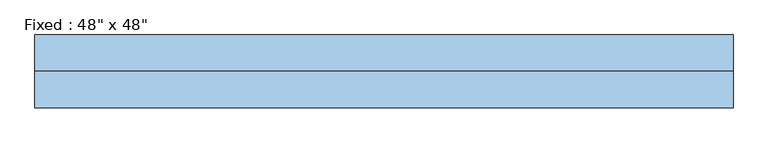
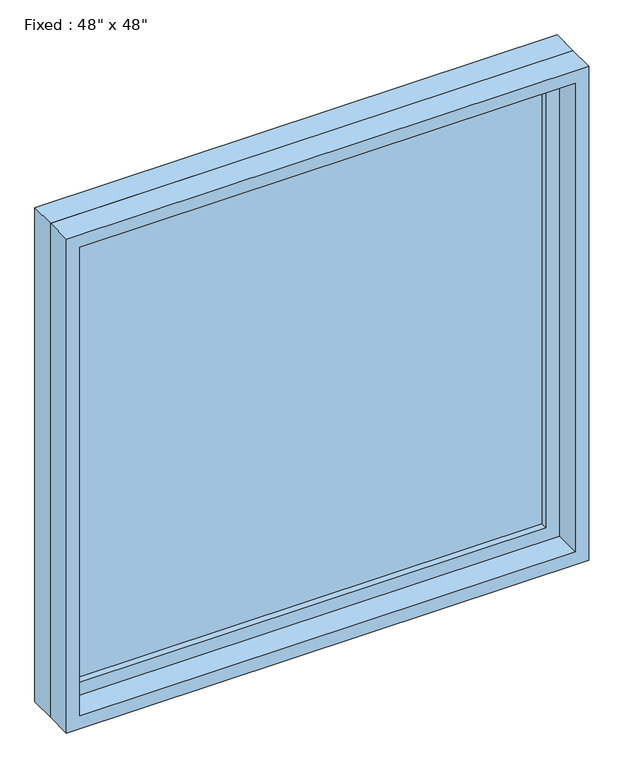
"""IFC4 building model written with IfcOpenShell, lengths in millimetres: window geometry."""

from ifc_helpers import new_model, si_unit, frame, origin, place, context, project, spatial, polyline, outline, extrude, source, transform, mapped, element, save


def window_f887c457(model_context):
    return source(origin(), model_context, "Body", "SweptSolid", [
        extrude(outline(polyline([(508.0, 15.875), (-584.2, 15.875), (-584.2, 28.575), (508.0, 28.575), (508.0, 15.875)])), frame((0.0, 0.0, 977.9), z_axis=(0.0, 0.0, 1.0), x_axis=(1.0, 0.0, 0.0)), (0.0, 0.0, 1.0), 1092.2),
        extrude(outline(polyline([(2114.55, -628.65), (933.45, -628.65), (933.45, 552.45), (2114.55, 552.45), (2114.55, -628.65)]), holes=[polyline([(2070.1, -584.2), (2070.1, 508.0), (977.9, 508.0), (977.9, -584.2), (2070.1, -584.2)])]), frame((0.0, 0.0, 0.0), z_axis=(0.0, 1.0, 0.0), x_axis=(0.0, 0.0, 1.0)), (0.0, 0.0, 1.0), 44.45),
        extrude(outline(polyline([(2133.6, -647.7), (914.4, -647.7), (914.4, 571.5), (2133.6, 571.5), (2133.6, -647.7)]), holes=[polyline([(2101.85, -615.95), (2101.85, 539.75), (946.15, 539.75), (946.15, -615.95), (2101.85, -615.95)])]), frame((0.0, -63.5, 0.0), z_axis=(0.0, 1.0, 0.0), x_axis=(0.0, 0.0, 1.0)), (0.0, 0.0, 1.0), 63.5),
        extrude(outline(polyline([(2133.6, 571.5), (2133.6, -647.7), (914.4, -647.7), (914.4, 571.5), (2133.6, 571.5)]), holes=[polyline([(2114.55, 552.45), (933.45, 552.45), (933.45, -628.65), (2114.55, -628.65), (2114.55, 552.45)])]), frame((0.0, 0.0, 0.0), z_axis=(0.0, 1.0, 0.0), x_axis=(0.0, 0.0, 1.0)), (0.0, 0.0, 1.0), 63.5),
    ])


if __name__ == "__main__":
    model = new_model("IFC4")
    model_context = context("Model", 3, world=origin())
    ifc_project = project(units=[si_unit("LENGTHUNIT", "METRE", prefix="MILLI")], contexts=[model_context])
    site = spatial("IfcSite", under=ifc_project)
    building = spatial("IfcBuilding", under=site)
    placement = place(None, origin())
    window_shape = window_f887c457(model_context)
    element("IfcWindow", 1, ObjectType="Fixed : 48\" x 48\"", at=placement, inside=building, context=model_context, shape_type="MappedRepresentation", body=[
        mapped(window_shape, transform((0.0, 0.0, 0.0), x_axis=(1.0, 0.0, 0.0), y_axis=(0.0, 1.0, 0.0), z_axis=(0.0, 0.0, 1.0))),
    ])
    save(model, "model.ifc")

# Revit data of these elements
# Type "Fixed : 48\" x 48\""
#   Type Mark = "2"
#   Assembly Code = "B2020100"
#   Height = 4' - 0"
#   Default Sill Height = 3' - 0"
#   Width = 4' - 0"
#   Window Inset = 0' - 0 3/4"
#   Glass Pane Material = Glass
#   Sash Material = Sash
#   Wall Closure = (empty or 0)
# Element 1 (IfcWindow, "Fixed : 48\" x 48\"")
#   Materials on its faces: "Sash", "Glass"
# Materials
#   "Glass": class "Glass", colour RGB 218 227 224, transparency 0.85, Description = "Soda Lime Glass", Cost = 0
#   "Sash": class "Wood", colour RGB 136 99 55, transparency 0
